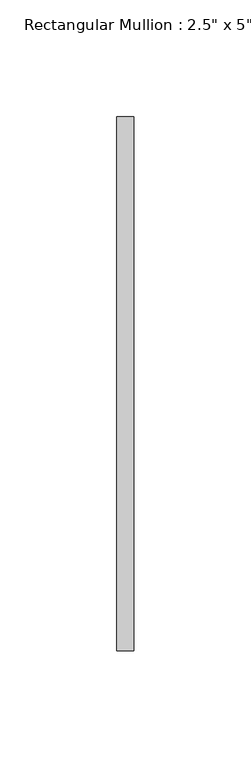
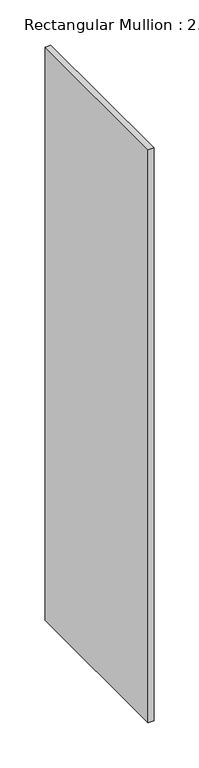
"""IFC4 building model written with IfcOpenShell, lengths in millimetres: member geometry."""

from ifc_helpers import new_model, si_unit, frame, origin, place, context, project, spatial, polyline, outline, extrude, source, transform, mapped, element, save


def member_2938acba(model_context):
    return source(origin(), model_context, "Body", "SweptSolid", [
        extrude(outline(polyline([(3.6195, 114.3), (3.6195, -114.3), (-3.6195, -114.3), (-3.6195, 114.3), (3.6195, 114.3)])), frame((0.0, 0.0, -774.7), z_axis=(0.0, 0.0, 1.0), x_axis=(1.0, 0.0, 0.0)), (0.0, 0.0, 1.0), 774.7),
    ])


if __name__ == "__main__":
    model = new_model("IFC4")
    model_context = context("Model", 3, world=origin())
    ifc_project = project(units=[si_unit("LENGTHUNIT", "METRE", prefix="MILLI")], contexts=[model_context])
    site = spatial("IfcSite", under=ifc_project)
    building = spatial("IfcBuilding", under=site)
    placement = place(None, origin())
    member_shape = member_2938acba(model_context)
    element("IfcMember", 1, ObjectType="Rectangular Mullion : 2.5\" x 5\" rectangular", at=placement, inside=building, context=model_context, shape_type="MappedRepresentation", body=[
        mapped(member_shape, transform((0.0, 0.0, 0.0), x_axis=(1.0, 0.0, 0.0), y_axis=(0.0, 1.0, 0.0), z_axis=(0.0, 0.0, 1.0))),
    ])
    save(model, "model.ifc")

# Revit data of these elements
# Type "Rectangular Mullion : 2.5\" x 5\" rectangular"
#   built-in parameter 1007304 = 0.75 (stored number, unit not read)
#   built-in parameter 1007301 = 0.011875 (stored number, unit not read)
#   built-in parameter 1007300 = 0.011875 (stored number, unit not read)
# Element 1 (IfcMember, "Rectangular Mullion : 2.5\" x 5\" rectangular")
#   Materials on its faces: "WINDOW GLASS MATERIAL"
# Materials
#   "WINDOW GLASS MATERIAL": class "Generic", colour RGB 120 120 120, transparency 0, Cost = 0
